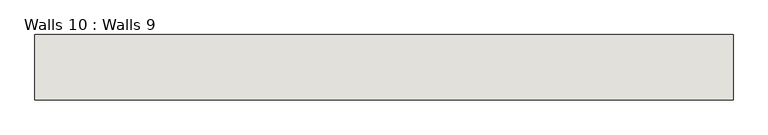
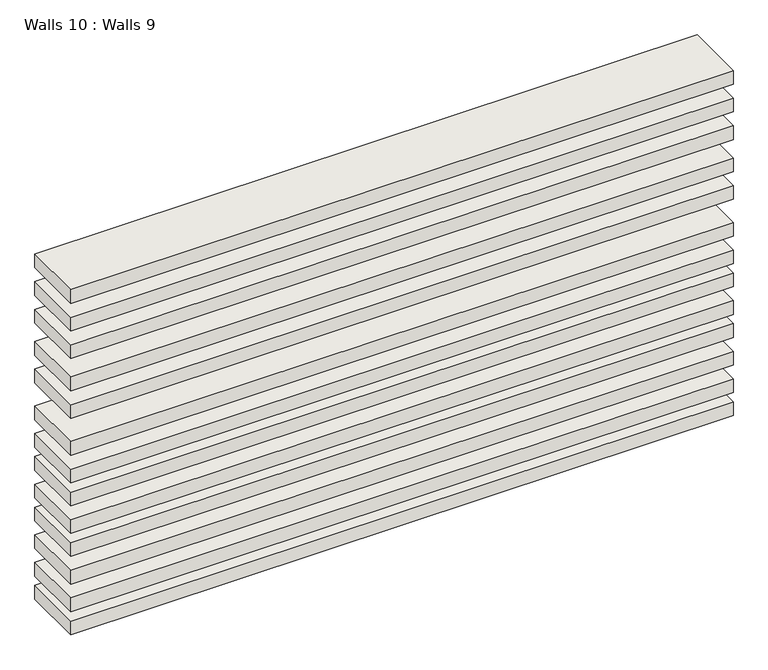
"""IFC4 building model written with IfcOpenShell, lengths in millimetres: wall geometry, Walls 10 : Walls 9."""

from ifc_helpers import new_model, si_unit, frame, origin, place, context, project, spatial, polyline, outline, extrude, source, transform, mapped, element, save


def walls_10_walls_9_f4ffd68b(model_context):
    return source(origin(), model_context, "Body", "SweptSolid", [
        extrude(outline(polyline([(77.6638712, -17646.2071125), (-3376.7361288, -17646.2071125), (-3376.7361288, -17322.090882), (77.6638712, -17322.090882), (77.6638712, -17646.2071125)])), frame((0.0, 0.0, 50.0), z_axis=(0.0, 0.0, 1.0), x_axis=(1.0, 0.0, 0.0)), (0.0, 0.0, 1.0), 75.9070443),
        extrude(outline(polyline([(77.6638712, -17646.2071125), (-3376.7361288, -17646.2071125), (-3376.7361288, -17322.090882), (77.6638712, -17322.090882), (77.6638712, -17646.2071125)])), frame((0.0, 0.0, 177.0), z_axis=(0.0, 0.0, 1.0), x_axis=(1.0, 0.0, 0.0)), (0.0, 0.0, 1.0), 75.9070443),
        extrude(outline(polyline([(77.6638712, -17646.2071125), (-3376.7361288, -17646.2071125), (-3376.7361288, -17322.090882), (77.6638712, -17322.090882), (77.6638712, -17646.2071125)])), frame((0.0, 0.0, 329.4), z_axis=(0.0, 0.0, 1.0), x_axis=(1.0, 0.0, 0.0)), (0.0, 0.0, 1.0), 75.9070443),
        extrude(outline(polyline([(77.6638712, -17646.2071125), (-3376.7361288, -17646.2071125), (-3376.7361288, -17322.090882), (77.6638712, -17322.090882), (77.6638712, -17646.2071125)])), frame((0.0, 0.0, 481.8), z_axis=(0.0, 0.0, 1.0), x_axis=(1.0, 0.0, 0.0)), (0.0, 0.0, 1.0), 75.9070443),
        extrude(outline(polyline([(77.6638712, -17646.2071125), (-3376.7361288, -17646.2071125), (-3376.7361288, -17322.090882), (77.6638712, -17322.090882), (77.6638712, -17646.2071125)])), frame((0.0, 0.0, 608.8), z_axis=(0.0, 0.0, 1.0), x_axis=(1.0, 0.0, 0.0)), (0.0, 0.0, 1.0), 75.9070443),
        extrude(outline(polyline([(77.6638712, -17646.2071125), (-3376.7361288, -17646.2071125), (-3376.7361288, -17322.090882), (77.6638712, -17322.090882), (77.6638712, -17646.2071125)])), frame((0.0, 0.0, 761.2), z_axis=(0.0, 0.0, 1.0), x_axis=(1.0, 0.0, 0.0)), (0.0, 0.0, 1.0), 75.9070443),
        extrude(outline(polyline([(77.6638712, -17646.2071125), (-3376.7361288, -17646.2071125), (-3376.7361288, -17322.090882), (77.6638712, -17322.090882), (77.6638712, -17646.2071125)])), frame((0.0, 0.0, 888.2), z_axis=(0.0, 0.0, 1.0), x_axis=(1.0, 0.0, 0.0)), (0.0, 0.0, 1.0), 75.9070443),
        extrude(outline(polyline([(77.6638712, -17646.2071125), (-3376.7361288, -17646.2071125), (-3376.7361288, -17322.090882), (77.6638712, -17322.090882), (77.6638712, -17646.2071125)])), frame((0.0, 0.0, 1040.6), z_axis=(0.0, 0.0, 1.0), x_axis=(1.0, 0.0, 0.0)), (0.0, 0.0, 1.0), 75.9070443),
        extrude(outline(polyline([(77.6638712, -17646.2071125), (-3376.7361288, -17646.2071125), (-3376.7361288, -17322.090882), (77.6638712, -17322.090882), (77.6638712, -17646.2071125)])), frame((0.0, 0.0, 1243.8), z_axis=(0.0, 0.0, 1.0), x_axis=(1.0, 0.0, 0.0)), (0.0, 0.0, 1.0), 75.9070443),
        extrude(outline(polyline([(77.6638712, -17646.2071125), (-3376.7361288, -17646.2071125), (-3376.7361288, -17322.090882), (77.6638712, -17322.090882), (77.6638712, -17646.2071125)])), frame((0.0, 0.0, 1396.2), z_axis=(0.0, 0.0, 1.0), x_axis=(1.0, 0.0, 0.0)), (0.0, 0.0, 1.0), 75.9070443),
        extrude(outline(polyline([(77.6638712, -17646.2071125), (-3376.7361288, -17646.2071125), (-3376.7361288, -17322.090882), (77.6638712, -17322.090882), (77.6638712, -17646.2071125)])), frame((0.0, 0.0, 1574.0), z_axis=(0.0, 0.0, 1.0), x_axis=(1.0, 0.0, 0.0)), (0.0, 0.0, 1.0), 75.9070443),
        extrude(outline(polyline([(77.6638712, -17646.2071125), (-3376.7361288, -17646.2071125), (-3376.7361288, -17322.090882), (77.6638712, -17322.090882), (77.6638712, -17646.2071125)])), frame((0.0, 0.0, 1726.4), z_axis=(0.0, 0.0, 1.0), x_axis=(1.0, 0.0, 0.0)), (0.0, 0.0, 1.0), 75.9070443),
        extrude(outline(polyline([(77.6638712, -17646.2071125), (-3376.7361288, -17646.2071125), (-3376.7361288, -17322.090882), (77.6638712, -17322.090882), (77.6638712, -17646.2071125)])), frame((0.0, 0.0, 1878.8), z_axis=(0.0, 0.0, 1.0), x_axis=(1.0, 0.0, 0.0)), (0.0, 0.0, 1.0), 75.9070443),
    ])


if __name__ == "__main__":
    model = new_model("IFC4")
    model_context = context("Model", 3, world=origin())
    ifc_project = project(units=[si_unit("LENGTHUNIT", "METRE", prefix="MILLI")], contexts=[model_context])
    site = spatial("IfcSite", under=ifc_project)
    building = spatial("IfcBuilding", under=site)
    placement = place(None, origin())
    walls_10_walls_9_shape = walls_10_walls_9_f4ffd68b(model_context)
    element("IfcWall", 1, ObjectType="Walls 10 : Walls 9", at=placement, inside=building, context=model_context, shape_type="MappedRepresentation", body=[
        mapped(walls_10_walls_9_shape, transform((0.0, 0.0, 0.0), x_axis=(1.0, 0.0, 0.0), y_axis=(0.0, 1.0, 0.0), z_axis=(0.0, 0.0, 1.0))),
    ])
    save(model, "model.ifc")

# Revit data of these elements
# Element 1 (IfcWall, "Walls 10 : Walls 9")
#   Materials on its faces: "Default Wall", "Door - Frame"
# Materials
#   "Default Wall": colour RGB 128 128 128, transparency 0
#   "Door - Frame": colour RGB 118 70 51, transparency 0
